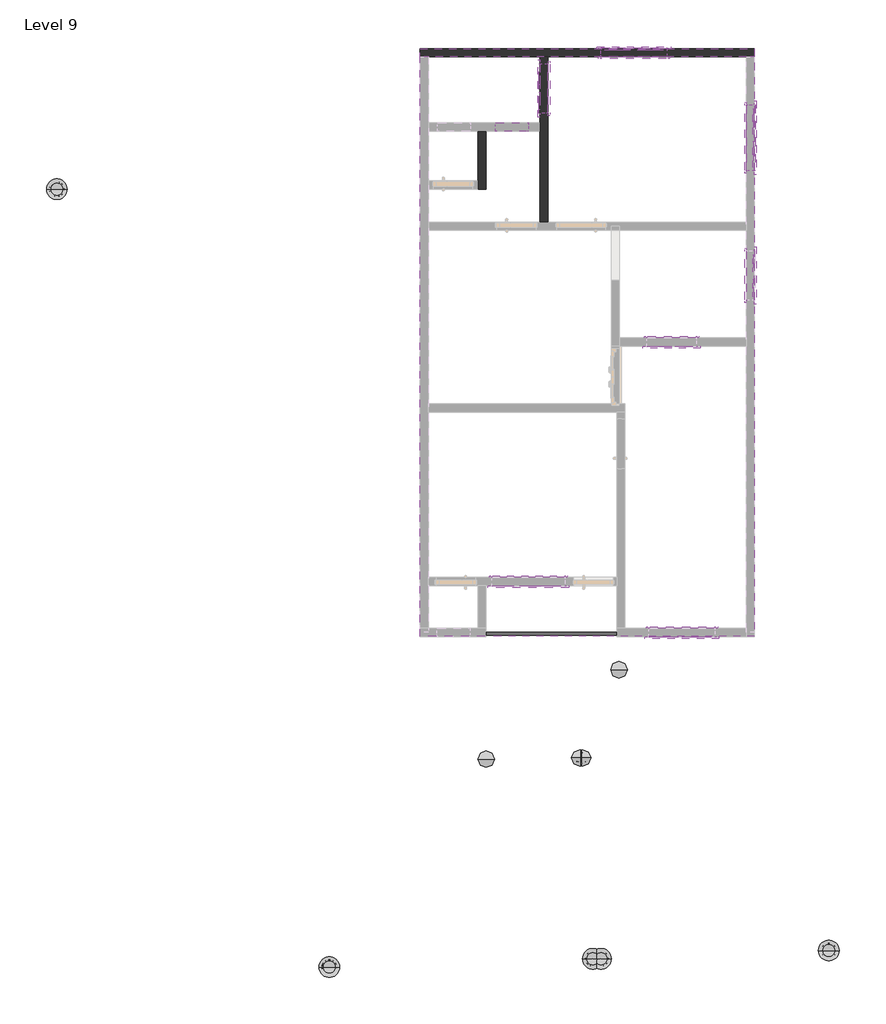
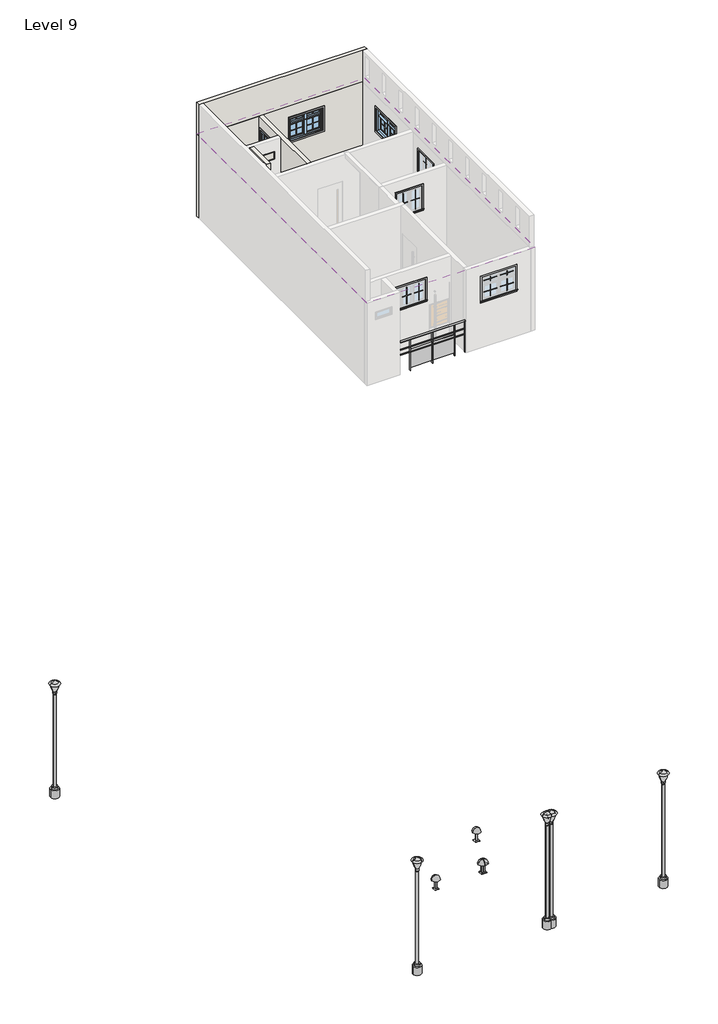
# One storey, part 2 of 2: 48 proxies, 10 light fixtures, 7 walls, 5 windows, 1 covering, 1 railing.
"""IFC4 building model written with IfcOpenShell, lengths in millimetres."""

from ifc_helpers import new_model, si_unit, point, frame, origin, place, context, project, spatial, polyline, ellipse_curve, trimmed, outline, extrude, faceted_brep, transform, mapped, element, save
from ifc_brep_helpers import plane_surface, extruded_surface, advanced_brep
from components import m_muntin_pattern_2x2_m_muntin_pattern_2x2_ec2ff75e, m_muntin_pattern_2x2_m_muntin_pattern_2x2_6a19bea2, m_muntin_pattern_2x2_m_muntin_pattern_2x2_383df7b3, m_muntin_pattern_2x2_m_muntin_pattern_2x2_55460d9e, m_muntin_pattern_2x2_m_muntin_pattern_2x2_a9b7b7a9, m_muntin_pattern_2x2_m_muntin_pattern_2x2_c959817e, m_muntin_pattern_2x2_m_muntin_pattern_2x2_9259c5e2, m_trim_window_exterior_flat_with_sill_b1b88069, m_trim_window_exterior_flat_with_sill_8fa486dc, m_trim_window_exterior_flat_with_sill_2a9c44ae, m_trim_window_interior_flat_picture_frame_7d12f20c, m_trim_window_interior_flat_picture_frame_b6dd03a6, m_trim_window_interior_flat_picture_frame_c139440e, m_street_light_antique_400w_halogen_120v_ac89fb25, m_table_lamp_hemispheric_60w_120v_fef6e77c, fixed_2_65c13adb, m_window_casement_double_3_e0bd8fa3, m_window_casement_double_awning_double_4_7efa9bbd

model = new_model("IFC4")

# Units and contexts
model_context = context("Model", 3, world=origin())
ifc_project = project(units=[si_unit("LENGTHUNIT", "METRE", prefix="MILLI")], contexts=[model_context])

# Site, building, storey
site = spatial("IfcSite", under=ifc_project)
building = spatial("IfcBuilding", under=site)
storey = spatial("IfcBuildingStorey", under=building, Name="Level 9", Elevation=16611.6)

# Proxies
placement = place(None, origin())
m_muntin_pattern_2x2_m_muntin_pattern_2x2_shape = m_muntin_pattern_2x2_m_muntin_pattern_2x2_ec2ff75e(model_context)
element("IfcBuildingElementProxy", 1, Name="M_Muntin Pattern_2x2 : M_Muntin Pattern_2x2", ObjectType="M_Muntin Pattern_2x2 : M_Muntin Pattern_2x2", at=placement, inside=storey, context=model_context, shape_type="MappedRepresentation", body=[
    mapped(m_muntin_pattern_2x2_m_muntin_pattern_2x2_shape, transform((-20164.8088079, 6316.5492053, 18510.25), x_axis=(1.0, 0.0, 0.0), y_axis=(0.0, 1.0, 0.0), z_axis=(0.0, 0.0, 1.0))),
])
element("IfcBuildingElementProxy", 2, Name="M_Muntin Pattern_2x2 : M_Muntin Pattern_2x2", ObjectType="M_Muntin Pattern_2x2 : M_Muntin Pattern_2x2", at=placement, inside=storey, context=model_context, shape_type="MappedRepresentation", body=[
    mapped(m_muntin_pattern_2x2_m_muntin_pattern_2x2_shape, transform((-17648.6213079, 4984.6367053, 18510.25), x_axis=(0.0, -1.0, 0.0), y_axis=(1.0, 0.0, 0.0), z_axis=(0.0, 0.0, 1.0))),
])
element("IfcBuildingElementProxy", 3, Name="M_Muntin Pattern_2x2 : M_Muntin Pattern_2x2", ObjectType="M_Muntin Pattern_2x2 : M_Muntin Pattern_2x2", at=placement, inside=storey, context=model_context, shape_type="MappedRepresentation", body=[
    mapped(m_muntin_pattern_2x2_m_muntin_pattern_2x2_shape, transform((-18672.7572454, -4510.2007947, 18510.25), x_axis=(-1.0, 0.0, 0.0), y_axis=(0.0, -1.0, 0.0), z_axis=(0.0, 0.0, 1.0))),
])
m_muntin_pattern_2x2_m_muntin_pattern_2x2_2_shape = m_muntin_pattern_2x2_m_muntin_pattern_2x2_6a19bea2(model_context)
element("IfcBuildingElementProxy", 4, Name="M_Muntin Pattern_2x2 : M_Muntin Pattern_2x2", ObjectType="M_Muntin Pattern_2x2 : M_Muntin Pattern_2x2", at=placement, inside=storey, context=model_context, shape_type="MappedRepresentation", body=[
    mapped(m_muntin_pattern_2x2_m_muntin_pattern_2x2_2_shape, transform((-19558.3838079, 6316.5492053, 18510.25), x_axis=(-1.0, 0.0, 0.0), y_axis=(0.0, -1.0, 0.0), z_axis=(0.0, 0.0, 1.0))),
])
element("IfcBuildingElementProxy", 5, Name="M_Muntin Pattern_2x2 : M_Muntin Pattern_2x2", ObjectType="M_Muntin Pattern_2x2 : M_Muntin Pattern_2x2", at=placement, inside=storey, context=model_context, shape_type="MappedRepresentation", body=[
    mapped(m_muntin_pattern_2x2_m_muntin_pattern_2x2_2_shape, transform((-17648.6213079, 4378.2117053, 18510.25), x_axis=(0.0, 1.0, 0.0), y_axis=(-1.0, 0.0, 0.0), z_axis=(0.0, 0.0, 1.0))),
])
element("IfcBuildingElementProxy", 6, Name="M_Muntin Pattern_2x2 : M_Muntin Pattern_2x2", ObjectType="M_Muntin Pattern_2x2 : M_Muntin Pattern_2x2", at=placement, inside=storey, context=model_context, shape_type="MappedRepresentation", body=[
    mapped(m_muntin_pattern_2x2_m_muntin_pattern_2x2_2_shape, transform((-19279.1822454, -4510.2007947, 18510.25), x_axis=(1.0, 0.0, 0.0), y_axis=(0.0, 1.0, 0.0), z_axis=(0.0, 0.0, 1.0))),
])
m_muntin_pattern_2x2_m_muntin_pattern_2x2_3_shape = m_muntin_pattern_2x2_m_muntin_pattern_2x2_383df7b3(model_context)
element("IfcBuildingElementProxy", 7, Name="M_Muntin Pattern_2x2 : M_Muntin Pattern_2x2", ObjectType="M_Muntin Pattern_2x2 : M_Muntin Pattern_2x2", at=placement, inside=storey, context=model_context, shape_type="MappedRepresentation", body=[
    mapped(m_muntin_pattern_2x2_m_muntin_pattern_2x2_3_shape, transform((-19558.3838079, 6316.5492053, 19110.25), x_axis=(-1.0, 0.0, 0.0), y_axis=(0.0, -1.0, 0.0), z_axis=(0.0, 0.0, 1.0))),
])
element("IfcBuildingElementProxy", 8, Name="M_Muntin Pattern_2x2 : M_Muntin Pattern_2x2", ObjectType="M_Muntin Pattern_2x2 : M_Muntin Pattern_2x2", at=placement, inside=storey, context=model_context, shape_type="MappedRepresentation", body=[
    mapped(m_muntin_pattern_2x2_m_muntin_pattern_2x2_3_shape, transform((-20164.8088079, 6316.5492053, 19110.25), x_axis=(-1.0, 0.0, 0.0), y_axis=(0.0, -1.0, 0.0), z_axis=(0.0, 0.0, 1.0))),
])
element("IfcBuildingElementProxy", 9, Name="M_Muntin Pattern_2x2 : M_Muntin Pattern_2x2", ObjectType="M_Muntin Pattern_2x2 : M_Muntin Pattern_2x2", at=placement, inside=storey, context=model_context, shape_type="MappedRepresentation", body=[
    mapped(m_muntin_pattern_2x2_m_muntin_pattern_2x2_3_shape, transform((-17648.6213079, 4378.2117053, 19110.25), x_axis=(0.0, 1.0, 0.0), y_axis=(-1.0, 0.0, 0.0), z_axis=(0.0, 0.0, 1.0))),
])
element("IfcBuildingElementProxy", 10, Name="M_Muntin Pattern_2x2 : M_Muntin Pattern_2x2", ObjectType="M_Muntin Pattern_2x2 : M_Muntin Pattern_2x2", at=placement, inside=storey, context=model_context, shape_type="MappedRepresentation", body=[
    mapped(m_muntin_pattern_2x2_m_muntin_pattern_2x2_3_shape, transform((-17648.6213079, 4984.6367053, 19110.25), x_axis=(0.0, 1.0, 0.0), y_axis=(-1.0, 0.0, 0.0), z_axis=(0.0, 0.0, 1.0))),
])
element("IfcBuildingElementProxy", 11, Name="M_Muntin Pattern_2x2 : M_Muntin Pattern_2x2", ObjectType="M_Muntin Pattern_2x2 : M_Muntin Pattern_2x2", at=placement, inside=storey, context=model_context, shape_type="MappedRepresentation", body=[
    mapped(m_muntin_pattern_2x2_m_muntin_pattern_2x2_3_shape, transform((-19279.1822454, -4510.2007947, 19110.25), x_axis=(1.0, 0.0, 0.0), y_axis=(0.0, 1.0, 0.0), z_axis=(0.0, 0.0, 1.0))),
])
element("IfcBuildingElementProxy", 12, Name="M_Muntin Pattern_2x2 : M_Muntin Pattern_2x2", ObjectType="M_Muntin Pattern_2x2 : M_Muntin Pattern_2x2", at=placement, inside=storey, context=model_context, shape_type="MappedRepresentation", body=[
    mapped(m_muntin_pattern_2x2_m_muntin_pattern_2x2_3_shape, transform((-18672.7572454, -4510.2007947, 19110.25), x_axis=(1.0, 0.0, 0.0), y_axis=(0.0, 1.0, 0.0), z_axis=(0.0, 0.0, 1.0))),
])
m_muntin_pattern_2x2_m_muntin_pattern_2x2_4_shape = m_muntin_pattern_2x2_m_muntin_pattern_2x2_55460d9e(model_context)
element("IfcBuildingElementProxy", 13, Name="M_Muntin Pattern_2x2 : M_Muntin Pattern_2x2", ObjectType="M_Muntin Pattern_2x2 : M_Muntin Pattern_2x2", at=placement, inside=storey, context=model_context, shape_type="MappedRepresentation", body=[
    mapped(m_muntin_pattern_2x2_m_muntin_pattern_2x2_4_shape, transform((-18939.9533391, 849.1992053, 18510.25), x_axis=(-1.0, 0.0, 0.0), y_axis=(0.0, -1.0, 0.0), z_axis=(0.0, 0.0, 1.0))),
])
element("IfcBuildingElementProxy", 14, Name="M_Muntin Pattern_2x2 : M_Muntin Pattern_2x2", ObjectType="M_Muntin Pattern_2x2 : M_Muntin Pattern_2x2", at=placement, inside=storey, context=model_context, shape_type="MappedRepresentation", body=[
    mapped(m_muntin_pattern_2x2_m_muntin_pattern_2x2_4_shape, transform((-17648.6213079, 2366.8492053, 18510.25), x_axis=(0.0, -1.0, 0.0), y_axis=(1.0, 0.0, 0.0), z_axis=(0.0, 0.0, 1.0))),
])
element("IfcBuildingElementProxy", 15, Name="M_Muntin Pattern_2x2 : M_Muntin Pattern_2x2", ObjectType="M_Muntin Pattern_2x2 : M_Muntin Pattern_2x2", at=placement, inside=storey, context=model_context, shape_type="MappedRepresentation", body=[
    mapped(m_muntin_pattern_2x2_m_muntin_pattern_2x2_4_shape, transform((-21591.9713079, 5362.4617053, 18510.25), x_axis=(0.0, 1.0, 0.0), y_axis=(-1.0, 0.0, 0.0), z_axis=(0.0, 0.0, 1.0))),
])
element("IfcBuildingElementProxy", 16, Name="M_Muntin Pattern_2x2 : M_Muntin Pattern_2x2", ObjectType="M_Muntin Pattern_2x2 : M_Muntin Pattern_2x2", at=placement, inside=storey, context=model_context, shape_type="MappedRepresentation", body=[
    mapped(m_muntin_pattern_2x2_m_muntin_pattern_2x2_4_shape, transform((-18939.9533391, 849.1992053, 18510.25), x_axis=(-1.0, 0.0, 0.0), y_axis=(0.0, -1.0, 0.0), z_axis=(0.0, 0.0, 1.0))),
])
element("IfcBuildingElementProxy", 17, Name="M_Muntin Pattern_2x2 : M_Muntin Pattern_2x2", ObjectType="M_Muntin Pattern_2x2 : M_Muntin Pattern_2x2", at=placement, inside=storey, context=model_context, shape_type="MappedRepresentation", body=[
    mapped(m_muntin_pattern_2x2_m_muntin_pattern_2x2_4_shape, transform((-21591.9713079, 5362.4617053, 18510.25), x_axis=(0.0, 1.0, 0.0), y_axis=(-1.0, 0.0, 0.0), z_axis=(0.0, 0.0, 1.0))),
])
m_muntin_pattern_2x2_m_muntin_pattern_2x2_5_shape = m_muntin_pattern_2x2_m_muntin_pattern_2x2_a9b7b7a9(model_context)
element("IfcBuildingElementProxy", 18, Name="M_Muntin Pattern_2x2 : M_Muntin Pattern_2x2", ObjectType="M_Muntin Pattern_2x2 : M_Muntin Pattern_2x2", at=placement, inside=storey, context=model_context, shape_type="MappedRepresentation", body=[
    mapped(m_muntin_pattern_2x2_m_muntin_pattern_2x2_5_shape, transform((-19393.9783391, 849.1992053, 18510.25), x_axis=(1.0, 0.0, 0.0), y_axis=(0.0, 1.0, 0.0), z_axis=(0.0, 0.0, 1.0))),
])
element("IfcBuildingElementProxy", 19, Name="M_Muntin Pattern_2x2 : M_Muntin Pattern_2x2", ObjectType="M_Muntin Pattern_2x2 : M_Muntin Pattern_2x2", at=placement, inside=storey, context=model_context, shape_type="MappedRepresentation", body=[
    mapped(m_muntin_pattern_2x2_m_muntin_pattern_2x2_5_shape, transform((-17648.6213079, 1912.8242053, 18510.25), x_axis=(0.0, 1.0, 0.0), y_axis=(-1.0, 0.0, 0.0), z_axis=(0.0, 0.0, 1.0))),
])
element("IfcBuildingElementProxy", 20, Name="M_Muntin Pattern_2x2 : M_Muntin Pattern_2x2", ObjectType="M_Muntin Pattern_2x2 : M_Muntin Pattern_2x2", at=placement, inside=storey, context=model_context, shape_type="MappedRepresentation", body=[
    mapped(m_muntin_pattern_2x2_m_muntin_pattern_2x2_5_shape, transform((-21591.9713079, 5816.4867053, 18510.25), x_axis=(0.0, -1.0, 0.0), y_axis=(1.0, 0.0, 0.0), z_axis=(0.0, 0.0, 1.0))),
])
element("IfcBuildingElementProxy", 21, Name="M_Muntin Pattern_2x2 : M_Muntin Pattern_2x2", ObjectType="M_Muntin Pattern_2x2 : M_Muntin Pattern_2x2", at=placement, inside=storey, context=model_context, shape_type="MappedRepresentation", body=[
    mapped(m_muntin_pattern_2x2_m_muntin_pattern_2x2_5_shape, transform((-19393.9783391, 849.1992053, 18510.25), x_axis=(1.0, 0.0, 0.0), y_axis=(0.0, 1.0, 0.0), z_axis=(0.0, 0.0, 1.0))),
])
element("IfcBuildingElementProxy", 22, Name="M_Muntin Pattern_2x2 : M_Muntin Pattern_2x2", ObjectType="M_Muntin Pattern_2x2 : M_Muntin Pattern_2x2", at=placement, inside=storey, context=model_context, shape_type="MappedRepresentation", body=[
    mapped(m_muntin_pattern_2x2_m_muntin_pattern_2x2_5_shape, transform((-21591.9713079, 5816.4867053, 18510.25), x_axis=(0.0, -1.0, 0.0), y_axis=(1.0, 0.0, 0.0), z_axis=(0.0, 0.0, 1.0))),
])
m_muntin_pattern_2x2_m_muntin_pattern_2x2_6_shape = m_muntin_pattern_2x2_m_muntin_pattern_2x2_c959817e(model_context)
element("IfcBuildingElementProxy", 23, Name="M_Muntin Pattern_2x2 : M_Muntin Pattern_2x2", ObjectType="M_Muntin Pattern_2x2 : M_Muntin Pattern_2x2", at=placement, inside=storey, context=model_context, shape_type="MappedRepresentation", body=[
    mapped(m_muntin_pattern_2x2_m_muntin_pattern_2x2_6_shape, transform((-21364.4296412, -3570.4007947, 18510.25), x_axis=(-1.0, 0.0, 0.0), y_axis=(0.0, -1.0, 0.0), z_axis=(0.0, 0.0, 1.0))),
])
element("IfcBuildingElementProxy", 24, Name="M_Muntin Pattern_2x2 : M_Muntin Pattern_2x2", ObjectType="M_Muntin Pattern_2x2 : M_Muntin Pattern_2x2", at=placement, inside=storey, context=model_context, shape_type="MappedRepresentation", body=[
    mapped(m_muntin_pattern_2x2_m_muntin_pattern_2x2_6_shape, transform((-21364.4296412, -3570.4007947, 18510.25), x_axis=(-1.0, 0.0, 0.0), y_axis=(0.0, -1.0, 0.0), z_axis=(0.0, 0.0, 1.0))),
])
m_muntin_pattern_2x2_m_muntin_pattern_2x2_7_shape = m_muntin_pattern_2x2_m_muntin_pattern_2x2_9259c5e2(model_context)
element("IfcBuildingElementProxy", 25, Name="M_Muntin Pattern_2x2 : M_Muntin Pattern_2x2", ObjectType="M_Muntin Pattern_2x2 : M_Muntin Pattern_2x2", at=placement, inside=storey, context=model_context, shape_type="MappedRepresentation", body=[
    mapped(m_muntin_pattern_2x2_m_muntin_pattern_2x2_7_shape, transform((-22257.6629746, -3570.4007947, 18510.25), x_axis=(1.0, 0.0, 0.0), y_axis=(0.0, 1.0, 0.0), z_axis=(0.0, 0.0, 1.0))),
])
element("IfcBuildingElementProxy", 26, Name="M_Muntin Pattern_2x2 : M_Muntin Pattern_2x2", ObjectType="M_Muntin Pattern_2x2 : M_Muntin Pattern_2x2", at=placement, inside=storey, context=model_context, shape_type="MappedRepresentation", body=[
    mapped(m_muntin_pattern_2x2_m_muntin_pattern_2x2_7_shape, transform((-21811.0463079, -3570.4007947, 18510.25), x_axis=(1.0, 0.0, 0.0), y_axis=(0.0, 1.0, 0.0), z_axis=(0.0, 0.0, 1.0))),
])
element("IfcBuildingElementProxy", 27, Name="M_Muntin Pattern_2x2 : M_Muntin Pattern_2x2", ObjectType="M_Muntin Pattern_2x2 : M_Muntin Pattern_2x2", at=placement, inside=storey, context=model_context, shape_type="MappedRepresentation", body=[
    mapped(m_muntin_pattern_2x2_m_muntin_pattern_2x2_7_shape, transform((-22257.6629746, -3570.4007947, 18510.25), x_axis=(1.0, 0.0, 0.0), y_axis=(0.0, 1.0, 0.0), z_axis=(0.0, 0.0, 1.0))),
])
element("IfcBuildingElementProxy", 28, Name="M_Muntin Pattern_2x2 : M_Muntin Pattern_2x2", ObjectType="M_Muntin Pattern_2x2 : M_Muntin Pattern_2x2", at=placement, inside=storey, context=model_context, shape_type="MappedRepresentation", body=[
    mapped(m_muntin_pattern_2x2_m_muntin_pattern_2x2_7_shape, transform((-21811.0463079, -3570.4007947, 18510.25), x_axis=(1.0, 0.0, 0.0), y_axis=(0.0, 1.0, 0.0), z_axis=(0.0, 0.0, 1.0))),
])
m_trim_window_exterior_flat_with_sill_shape = m_trim_window_exterior_flat_with_sill_b1b88069(model_context)
element("IfcBuildingElementProxy", 29, Name="M_Trim-Window-Exterior-Flat : with Sill", ObjectType="M_Trim-Window-Exterior-Flat : with Sill", at=placement, inside=storey, context=model_context, shape_type="MappedRepresentation", body=[
    mapped(m_trim_window_exterior_flat_with_sill_shape, transform((-19861.5963079, 6326.0742053, 19340.4), x_axis=(-1.0, 0.0, 0.0), y_axis=(0.0, 0.0, 1.0), z_axis=(0.0, 1.0, 0.0))),
])
element("IfcBuildingElementProxy", 30, Name="M_Trim-Window-Exterior-Flat : with Sill", ObjectType="M_Trim-Window-Exterior-Flat : with Sill", at=placement, inside=storey, context=model_context, shape_type="MappedRepresentation", body=[
    mapped(m_trim_window_exterior_flat_with_sill_shape, transform((-17639.0963079, 4681.4242053, 19340.4), x_axis=(0.0, 1.0, 0.0), y_axis=(0.0, 0.0, 1.0), z_axis=(1.0, 0.0, 0.0))),
])
element("IfcBuildingElementProxy", 31, Name="M_Trim-Window-Exterior-Flat : with Sill", ObjectType="M_Trim-Window-Exterior-Flat : with Sill", at=placement, inside=storey, context=model_context, shape_type="MappedRepresentation", body=[
    mapped(m_trim_window_exterior_flat_with_sill_shape, transform((-18975.9697454, -4519.7257947, 19340.4), x_axis=(1.0, 0.0, 0.0), y_axis=(0.0, 0.0, 1.0), z_axis=(0.0, -1.0, 0.0))),
])
m_trim_window_exterior_flat_with_sill_2_shape = m_trim_window_exterior_flat_with_sill_8fa486dc(model_context)
element("IfcBuildingElementProxy", 32, Name="M_Trim-Window-Exterior-Flat : with Sill", ObjectType="M_Trim-Window-Exterior-Flat : with Sill", at=placement, inside=storey, context=model_context, shape_type="MappedRepresentation", body=[
    mapped(m_trim_window_exterior_flat_with_sill_2_shape, transform((-19166.9658391, 839.6742053, 19340.4), x_axis=(1.0, 0.0, 0.0), y_axis=(0.0, 0.0, 1.0), z_axis=(0.0, -1.0, 0.0))),
])
element("IfcBuildingElementProxy", 33, Name="M_Trim-Window-Exterior-Flat : with Sill", ObjectType="M_Trim-Window-Exterior-Flat : with Sill", at=placement, inside=storey, context=model_context, shape_type="MappedRepresentation", body=[
    mapped(m_trim_window_exterior_flat_with_sill_2_shape, transform((-17639.0963079, 2139.8367053, 19340.4), x_axis=(0.0, 1.0, 0.0), y_axis=(0.0, 0.0, 1.0), z_axis=(1.0, 0.0, 0.0))),
])
element("IfcBuildingElementProxy", 34, Name="M_Trim-Window-Exterior-Flat : with Sill", ObjectType="M_Trim-Window-Exterior-Flat : with Sill", at=placement, inside=storey, context=model_context, shape_type="MappedRepresentation", body=[
    mapped(m_trim_window_exterior_flat_with_sill_2_shape, transform((-21601.4963079, 5589.4742053, 19340.4), x_axis=(0.0, -1.0, 0.0), y_axis=(0.0, 0.0, 1.0), z_axis=(-1.0, 0.0, 0.0))),
])
element("IfcBuildingElementProxy", 35, Name="M_Trim-Window-Exterior-Flat : with Sill", ObjectType="M_Trim-Window-Exterior-Flat : with Sill", at=placement, inside=storey, context=model_context, shape_type="MappedRepresentation", body=[
    mapped(m_trim_window_exterior_flat_with_sill_2_shape, transform((-19166.9658391, 839.6742053, 19340.4), x_axis=(1.0, 0.0, 0.0), y_axis=(0.0, 0.0, 1.0), z_axis=(0.0, -1.0, 0.0))),
])
element("IfcBuildingElementProxy", 36, Name="M_Trim-Window-Exterior-Flat : with Sill", ObjectType="M_Trim-Window-Exterior-Flat : with Sill", at=placement, inside=storey, context=model_context, shape_type="MappedRepresentation", body=[
    mapped(m_trim_window_exterior_flat_with_sill_2_shape, transform((-21601.4963079, 5589.4742053, 19340.4), x_axis=(0.0, -1.0, 0.0), y_axis=(0.0, 0.0, 1.0), z_axis=(-1.0, 0.0, 0.0))),
])
m_trim_window_exterior_flat_with_sill_3_shape = m_trim_window_exterior_flat_with_sill_2a9c44ae(model_context)
element("IfcBuildingElementProxy", 37, Name="M_Trim-Window-Exterior-Flat : with Sill", ObjectType="M_Trim-Window-Exterior-Flat : with Sill", at=placement, inside=storey, context=model_context, shape_type="MappedRepresentation", body=[
    mapped(m_trim_window_exterior_flat_with_sill_3_shape, transform((-21811.0463079, -3579.9257947, 19240.4), x_axis=(1.0, 0.0, 0.0), y_axis=(0.0, 0.0, 1.0), z_axis=(0.0, -1.0, 0.0))),
])
element("IfcBuildingElementProxy", 38, Name="M_Trim-Window-Exterior-Flat : with Sill", ObjectType="M_Trim-Window-Exterior-Flat : with Sill", at=placement, inside=storey, context=model_context, shape_type="MappedRepresentation", body=[
    mapped(m_trim_window_exterior_flat_with_sill_3_shape, transform((-21811.0463079, -3579.9257947, 19240.4), x_axis=(1.0, 0.0, 0.0), y_axis=(0.0, 0.0, 1.0), z_axis=(0.0, -1.0, 0.0))),
])
m_trim_window_interior_flat_picture_frame_shape = m_trim_window_interior_flat_picture_frame_7d12f20c(model_context)
element("IfcBuildingElementProxy", 39, Name="M_Trim-Window-Interior-Flat : Picture Frame", ObjectType="M_Trim-Window-Interior-Flat : Picture Frame", at=placement, inside=storey, context=model_context, shape_type="MappedRepresentation", body=[
    mapped(m_trim_window_interior_flat_picture_frame_shape, transform((-19861.5963079, 6173.6742053, 19340.4), x_axis=(1.0, 0.0, 0.0), y_axis=(0.0, 0.0, 1.0), z_axis=(0.0, -1.0, 0.0))),
])
element("IfcBuildingElementProxy", 40, Name="M_Trim-Window-Interior-Flat : Picture Frame", ObjectType="M_Trim-Window-Interior-Flat : Picture Frame", at=placement, inside=storey, context=model_context, shape_type="MappedRepresentation", body=[
    mapped(m_trim_window_interior_flat_picture_frame_shape, transform((-17791.4963079, 4681.4242053, 19340.4), x_axis=(0.0, -1.0, 0.0), y_axis=(0.0, 0.0, 1.0), z_axis=(-1.0, 0.0, 0.0))),
])
element("IfcBuildingElementProxy", 41, Name="M_Trim-Window-Interior-Flat : Picture Frame", ObjectType="M_Trim-Window-Interior-Flat : Picture Frame", at=placement, inside=storey, context=model_context, shape_type="MappedRepresentation", body=[
    mapped(m_trim_window_interior_flat_picture_frame_shape, transform((-18975.9697454, -4367.3257947, 19340.4), x_axis=(-1.0, 0.0, 0.0), y_axis=(0.0, 0.0, 1.0), z_axis=(0.0, 1.0, 0.0))),
])
m_trim_window_interior_flat_picture_frame_2_shape = m_trim_window_interior_flat_picture_frame_b6dd03a6(model_context)
element("IfcBuildingElementProxy", 42, Name="M_Trim-Window-Interior-Flat : Picture Frame", ObjectType="M_Trim-Window-Interior-Flat : Picture Frame", at=placement, inside=storey, context=model_context, shape_type="MappedRepresentation", body=[
    mapped(m_trim_window_interior_flat_picture_frame_2_shape, transform((-19166.9658391, 992.0742053, 19340.4), x_axis=(-1.0, 0.0, 0.0), y_axis=(0.0, 0.0, 1.0), z_axis=(0.0, 1.0, 0.0))),
])
element("IfcBuildingElementProxy", 43, Name="M_Trim-Window-Interior-Flat : Picture Frame", ObjectType="M_Trim-Window-Interior-Flat : Picture Frame", at=placement, inside=storey, context=model_context, shape_type="MappedRepresentation", body=[
    mapped(m_trim_window_interior_flat_picture_frame_2_shape, transform((-17791.4963079, 2139.8367053, 19340.4), x_axis=(0.0, -1.0, 0.0), y_axis=(0.0, 0.0, 1.0), z_axis=(-1.0, 0.0, 0.0))),
])
element("IfcBuildingElementProxy", 44, Name="M_Trim-Window-Interior-Flat : Picture Frame", ObjectType="M_Trim-Window-Interior-Flat : Picture Frame", at=placement, inside=storey, context=model_context, shape_type="MappedRepresentation", body=[
    mapped(m_trim_window_interior_flat_picture_frame_2_shape, transform((-21449.0963079, 5589.4742053, 19340.4), x_axis=(0.0, 1.0, 0.0), y_axis=(0.0, 0.0, 1.0), z_axis=(1.0, 0.0, 0.0))),
])
element("IfcBuildingElementProxy", 45, Name="M_Trim-Window-Interior-Flat : Picture Frame", ObjectType="M_Trim-Window-Interior-Flat : Picture Frame", at=placement, inside=storey, context=model_context, shape_type="MappedRepresentation", body=[
    mapped(m_trim_window_interior_flat_picture_frame_2_shape, transform((-19166.9658391, 992.0742053, 19340.4), x_axis=(-1.0, 0.0, 0.0), y_axis=(0.0, 0.0, 1.0), z_axis=(0.0, 1.0, 0.0))),
])
element("IfcBuildingElementProxy", 46, Name="M_Trim-Window-Interior-Flat : Picture Frame", ObjectType="M_Trim-Window-Interior-Flat : Picture Frame", at=placement, inside=storey, context=model_context, shape_type="MappedRepresentation", body=[
    mapped(m_trim_window_interior_flat_picture_frame_2_shape, transform((-21449.0963079, 5589.4742053, 19340.4), x_axis=(0.0, 1.0, 0.0), y_axis=(0.0, 0.0, 1.0), z_axis=(1.0, 0.0, 0.0))),
])
m_trim_window_interior_flat_picture_frame_3_shape = m_trim_window_interior_flat_picture_frame_c139440e(model_context)
element("IfcBuildingElementProxy", 47, Name="M_Trim-Window-Interior-Flat : Picture Frame", ObjectType="M_Trim-Window-Interior-Flat : Picture Frame", at=placement, inside=storey, context=model_context, shape_type="MappedRepresentation", body=[
    mapped(m_trim_window_interior_flat_picture_frame_3_shape, transform((-21811.0463079, -3427.5257947, 19240.4), x_axis=(-1.0, 0.0, 0.0), y_axis=(0.0, 0.0, 1.0), z_axis=(0.0, 1.0, 0.0))),
])
element("IfcBuildingElementProxy", 48, Name="M_Trim-Window-Interior-Flat : Picture Frame", ObjectType="M_Trim-Window-Interior-Flat : Picture Frame", at=placement, inside=storey, context=model_context, shape_type="MappedRepresentation", body=[
    mapped(m_trim_window_interior_flat_picture_frame_3_shape, transform((-21811.0463079, -3427.5257947, 19240.4), x_axis=(-1.0, 0.0, 0.0), y_axis=(0.0, 0.0, 1.0), z_axis=(0.0, 1.0, 0.0))),
])

# Covering
element("IfcCovering", 49, ObjectType="2' x 4' ACT System", at=placement, inside=storey, context=model_context, shape_type="SweptSolid", body=[
    extrude(outline(polyline([(-23811.2963079, -4519.7257947), (-23811.2963079, 6326.0742053), (-17639.0963079, 6326.0742053), (-17639.0963079, -4519.7257947), (-22309.2664727, -4519.7257947), (-23811.2963079, -4519.7257947)])), frame((0.0, 0.0, 19812.0), z_axis=(0.0, 0.0, 1.0), x_axis=(1.0, 0.0, 0.0)), (0.0, 0.0, 1.0), 57.15),
])

# Light fixtures
m_street_light_antique_400w_halogen_120v_shape = m_street_light_antique_400w_halogen_120v_ac89fb25(model_context)
element("IfcLightFixture", 50, ObjectType="M_Street Light - Antique : 400W Halogen - 120V", at=placement, inside=storey, context=model_context, shape_type="MappedRepresentation", body=[
    mapped(m_street_light_antique_400w_halogen_120v_shape, transform((-16267.4963079, -10310.2685721, -1936.0232956), x_axis=(1.0, 0.0, 0.0), y_axis=(0.0, 1.0, 0.0), z_axis=(0.0, 0.0, 1.0))),
])
element("IfcLightFixture", 51, ObjectType="M_Street Light - Antique : 400W Halogen - 120V", at=placement, inside=storey, context=model_context, shape_type="MappedRepresentation", body=[
    mapped(m_street_light_antique_400w_halogen_120v_shape, transform((-20471.1963079, -10462.8323892, -1917.9019302), x_axis=(1.0, 0.0, 0.0), y_axis=(0.0, 1.0, 0.0), z_axis=(0.0, 0.0, 1.0))),
])
element("IfcLightFixture", 52, ObjectType="M_Street Light - Antique : 400W Halogen - 120V", at=placement, inside=storey, context=model_context, shape_type="MappedRepresentation", body=[
    mapped(m_street_light_antique_400w_halogen_120v_shape, transform((-20623.5963079, -10462.8323892, -1917.9019302), x_axis=(1.0, 0.0, 0.0), y_axis=(0.0, 1.0, 0.0), z_axis=(0.0, 0.0, 1.0))),
])
element("IfcLightFixture", 53, ObjectType="M_Street Light - Antique : 400W Halogen - 120V", at=placement, inside=storey, context=model_context, shape_type="MappedRepresentation", body=[
    mapped(m_street_light_antique_400w_halogen_120v_shape, transform((-25487.6963079, -10615.7175512, -1899.7423958), x_axis=(1.0, 0.0, 0.0), y_axis=(0.0, 1.0, 0.0), z_axis=(0.0, 0.0, 1.0))),
])
element("IfcLightFixture", 54, ObjectType="M_Street Light - Antique : 400W Halogen - 120V", at=placement, inside=storey, context=model_context, shape_type="MappedRepresentation", body=[
    mapped(m_street_light_antique_400w_halogen_120v_shape, transform((-30516.8963079, 3735.2742053, -1981.2), x_axis=(1.0, 0.0, 0.0), y_axis=(0.0, 1.0, 0.0), z_axis=(0.0, 0.0, 1.0))),
])
m_table_lamp_hemispheric_60w_120v_shape = m_table_lamp_hemispheric_60w_120v_fef6e77c(model_context)
element("IfcLightFixture", 55, ObjectType="M_Table Lamp - Hemispheric : 60W - 120V", at=placement, inside=storey, context=model_context, shape_type="MappedRepresentation", body=[
    mapped(m_table_lamp_hemispheric_60w_120v_shape, transform((-22592.0963079, -6780.3257947, -1981.2), x_axis=(1.0, 0.0, 0.0), y_axis=(0.0, 1.0, 0.0), z_axis=(0.0, 0.0, 1.0))),
])
element("IfcLightFixture", 56, ObjectType="M_Table Lamp - Hemispheric : 60W - 120V", at=placement, inside=storey, context=model_context, shape_type="MappedRepresentation", body=[
    mapped(m_table_lamp_hemispheric_60w_120v_shape, transform((-20864.8963079, -6754.9257947, -1981.2), x_axis=(1.0, 0.0, 0.0), y_axis=(0.0, 1.0, 0.0), z_axis=(0.0, 0.0, 1.0))),
])
element("IfcLightFixture", 57, ObjectType="M_Table Lamp - Hemispheric : 60W - 120V", at=placement, inside=storey, context=model_context, shape_type="MappedRepresentation", body=[
    mapped(m_table_lamp_hemispheric_60w_120v_shape, transform((-20814.0963079, -6754.9257947, -1981.2), x_axis=(1.0, 0.0, 0.0), y_axis=(0.0, 1.0, 0.0), z_axis=(0.0, 0.0, 1.0))),
])
element("IfcLightFixture", 58, ObjectType="M_Table Lamp - Hemispheric : 60W - 120V", at=placement, inside=storey, context=model_context, shape_type="MappedRepresentation", body=[
    mapped(m_table_lamp_hemispheric_60w_120v_shape, transform((-20839.4963079, -6754.9257947, -1981.2), x_axis=(1.0, 0.0, 0.0), y_axis=(0.0, 1.0, 0.0), z_axis=(0.0, 0.0, 1.0))),
])
element("IfcLightFixture", 59, ObjectType="M_Table Lamp - Hemispheric : 60W - 120V", at=placement, inside=storey, context=model_context, shape_type="MappedRepresentation", body=[
    mapped(m_table_lamp_hemispheric_60w_120v_shape, transform((-20140.9963079, -5129.3257947, -1981.2), x_axis=(1.0, 0.0, 0.0), y_axis=(0.0, 1.0, 0.0), z_axis=(0.0, 0.0, 1.0))),
])

# Railing
element("IfcRailing", 60, ObjectType="Glass Panel - Bottom Fill", at=placement, inside=storey, context=model_context, shape_type="SolidModel", body=[
    advanced_brep(
    [(-22592.0963079, -4430.8257947, 17830.8), (-22592.0963079, -4507.0257947, 17830.8), (-20179.0963079, -4430.8257947, 17830.8), (-20179.0963079, -4507.0257947, 17830.8)],
    [
        (0, 1, ellipse_curve(frame((-22592.0963079, -4468.9257947, 17830.8), z_axis=(-1.0, 0.0, 0.0), x_axis=(0.0, -1.0, 0.0)), 38.1, 28.575)),
        (1, 0, ellipse_curve(frame((-22592.0963079, -4468.9257947, 17830.8), z_axis=(-1.0, 0.0, 0.0), x_axis=(0.0, -1.0, 0.0)), 38.1, 28.575)),
        (2, 3, ellipse_curve(frame((-20179.0963079, -4468.9257947, 17830.8), z_axis=(1.0, 0.0, 0.0), x_axis=(0.0, -1.0, 0.0)), 38.1, 28.575)),
        (3, 2, ellipse_curve(frame((-20179.0963079, -4468.9257947, 17830.8), z_axis=(1.0, 0.0, 0.0), x_axis=(0.0, -1.0, 0.0)), 38.1, 28.575)),
        (0, 2),
        (3, 1),
    ],
    [
        plane_surface(frame((-22592.0963079, -4468.9257947, 17830.8), z_axis=(-1.0, 0.0, 0.0), x_axis=(0.0, 1.0, 0.0))),
        plane_surface(frame((-20179.0963079, -4468.9257947, 17830.8), z_axis=(1.0, 0.0, 0.0), x_axis=(0.0, 1.0, 0.0))),
        extruded_surface(trimmed(ellipse_curve(frame((-20179.0963079, -4468.9257947, 17830.8), z_axis=(-1.0, 0.0, 0.0), x_axis=(0.0, -1.0, 0.0)), 38.1, 28.575), [point((-20179.0963079, -4430.8257947, 17830.8))], [point((-20179.0963079, -4507.0257947, 17830.8))], True, "CARTESIAN"), (-2413.0, 0.0, 0.0), 2413.0),
        extruded_surface(trimmed(ellipse_curve(frame((-20179.0963079, -4468.9257947, 17830.8), z_axis=(-1.0, 0.0, 0.0), x_axis=(0.0, -1.0, 0.0)), 38.1, 28.575), [point((-20179.0963079, -4507.0257947, 17830.8))], [point((-20179.0963079, -4430.8257947, 17830.8))], True, "CARTESIAN"), (-2413.0, 0.0, 0.0), 2413.0),
    ],
    [
        (0, [[1, 2]]),
        (1, [[3, 4]]),
        (2, [[-1, 5, -4, 6]]),
        (3, [[-2, -6, -3, -5]]),
    ],
),
    extrude(outline(polyline([(-22592.0963079, -4481.6257947), (-22592.0963079, -4456.2257947), (-20179.0963079, -4456.2257947), (-20179.0963079, -4481.6257947), (-22592.0963079, -4481.6257947)])), frame((0.0, 0.0, 17513.3), z_axis=(0.0, 0.0, 1.0), x_axis=(1.0, 0.0, 0.0)), (0.0, 0.0, 1.0), 25.4),
    extrude(outline(polyline([(-22592.0963079, -4481.6257947), (-22592.0963079, -4456.2257947), (-20179.0963079, -4456.2257947), (-20179.0963079, -4481.6257947), (-22592.0963079, -4481.6257947)])), frame((0.0, 0.0, 17310.1), z_axis=(0.0, 0.0, 1.0), x_axis=(1.0, 0.0, 0.0)), (0.0, 0.0, 1.0), 25.4),
    extrude(outline(polyline([(-20579.1463079, -4494.3257947), (-20579.1463079, -4443.5257947), (-20566.4463079, -4443.5257947), (-20566.4463079, -4494.3257947), (-20579.1463079, -4494.3257947)])), frame((0.0, 0.0, 16611.6), z_axis=(0.0, 0.0, 1.0), x_axis=(1.0, 0.0, 0.0)), (0.0, 0.0, 1.0), 1190.625),
    extrude(outline(polyline([(-21385.5963079, -4462.3906377), (-20572.7963079, -4462.3906377), (-20572.7963079, -4468.7406377), (-21385.5963079, -4468.7406377), (-21385.5963079, -4462.3906377)])), frame((0.0, 0.0, 16713.2), z_axis=(0.0, 0.0, 1.0), x_axis=(1.0, 0.0, 0.0)), (0.0, 0.0, 1.0), 711.2),
    extrude(outline(polyline([(-21391.9463079, -4494.3257947), (-21391.9463079, -4443.5257947), (-21379.2463079, -4443.5257947), (-21379.2463079, -4494.3257947), (-21391.9463079, -4494.3257947)])), frame((0.0, 0.0, 16611.6), z_axis=(0.0, 0.0, 1.0), x_axis=(1.0, 0.0, 0.0)), (0.0, 0.0, 1.0), 1190.625),
    extrude(outline(polyline([(-22198.3963079, -4462.3906377), (-21385.5963079, -4462.3906377), (-21385.5963079, -4468.7406377), (-22198.3963079, -4468.7406377), (-22198.3963079, -4462.3906377)])), frame((0.0, 0.0, 16713.2), z_axis=(0.0, 0.0, 1.0), x_axis=(1.0, 0.0, 0.0)), (0.0, 0.0, 1.0), 711.2),
    extrude(outline(polyline([(-22204.7463079, -4494.3257947), (-22204.7463079, -4443.5257947), (-22192.0463079, -4443.5257947), (-22192.0463079, -4494.3257947), (-22204.7463079, -4494.3257947)])), frame((0.0, 0.0, 16611.6), z_axis=(0.0, 0.0, 1.0), x_axis=(1.0, 0.0, 0.0)), (0.0, 0.0, 1.0), 1190.625),
    extrude(outline(polyline([(-20191.7963079, -4478.4507947), (-20191.7963079, -4459.4007947), (-20172.7463079, -4459.4007947), (-20172.7463079, -4478.4507947), (-20191.7963079, -4478.4507947)])), frame((0.0, 0.0, 16611.6), z_axis=(0.0, 0.0, 1.0), x_axis=(1.0, 0.0, 0.0)), (0.0, 0.0, 1.0), 1190.625),
    extrude(outline(polyline([(-22598.4463079, -4478.4507947), (-22598.4463079, -4459.4007947), (-22579.3963079, -4459.4007947), (-22579.3963079, -4478.4507947), (-22598.4463079, -4478.4507947)])), frame((0.0, 0.0, 16611.6), z_axis=(0.0, 0.0, 1.0), x_axis=(1.0, 0.0, 0.0)), (0.0, 0.0, 1.0), 1190.625),
])

# Walls
element("IfcWall", 61, ObjectType="Generic - 6\"", at=placement, inside=storey, context=model_context, shape_type="Brep", body=[
    faceted_brep([(-23811.2963079, 6173.6742053, 16611.6), (-23658.8963079, 6173.6742053, 16611.6), (-21601.4963079, 6173.6742053, 16611.6), (-21449.0963079, 6173.6742053, 16611.6), (-17791.4963079, 6173.6742053, 16611.6), (-17639.0963079, 6173.6742053, 16611.6), (-17639.0963079, 6173.6742053, 19812.0), (-17791.4963079, 6173.6742053, 19812.0), (-21449.0963079, 6173.6742053, 19812.0), (-21601.4963079, 6173.6742053, 19812.0), (-23658.8963079, 6173.6742053, 19812.0), (-23811.2963079, 6173.6742053, 19812.0), (-19251.9963079, 6173.6742053, 19340.4), (-19251.9963079, 6173.6742053, 18440.4), (-20471.1963079, 6173.6742053, 18440.4), (-20471.1963079, 6173.6742053, 19340.4), (-23811.2963079, 6326.0742053, 16611.6), (-23811.2963079, 6326.0742053, 19812.0), (-17639.0963079, 6326.0742053, 19812.0), (-17639.0963079, 6326.0742053, 16611.6), (-19251.9963079, 6326.0742053, 19340.4), (-20471.1963079, 6326.0742053, 19340.4), (-20471.1963079, 6326.0742053, 18440.4), (-19251.9963079, 6326.0742053, 18440.4)], [[[0, 1, 2, 3, 4, 5, 6, 7, 8, 9, 10, 11], [12, 13, 14, 15]], [[16, 17, 18, 19], [20, 21, 22, 23]], [[5, 4, 3, 2, 1, 0, 16, 19]], [[11, 10, 9, 8, 7, 6, 18, 17]], [[6, 5, 19, 18]], [[0, 11, 17, 16]], [[13, 12, 20, 23]], [[14, 13, 23, 22]], [[15, 14, 22, 21]], [[12, 15, 21, 20]]]),
])
element("IfcWall", 62, ObjectType="Generic - 6\"", at=placement, inside=storey, context=model_context, shape_type="Brep", body=[
    faceted_brep([(-21601.4963079, 6173.6742053, 16611.6), (-21601.4963079, 4954.4742053, 16611.6), (-21601.4963079, 4802.0742053, 16611.6), (-21601.4963079, 3125.6742053, 16611.6), (-21601.4963079, 3125.6742053, 19812.0), (-21601.4963079, 4802.0742053, 19812.0), (-21601.4963079, 4954.4742053, 19812.0), (-21601.4963079, 6173.6742053, 19812.0), (-21601.4963079, 6046.6742053, 19340.4), (-21601.4963079, 5132.2742053, 19340.4), (-21601.4963079, 5132.2742053, 18440.4), (-21601.4963079, 6046.6742053, 18440.4), (-21449.0963079, 6173.6742053, 16611.6), (-21449.0963079, 6173.6742053, 19812.0), (-21449.0963079, 3125.6742053, 19812.0), (-21449.0963079, 3125.6742053, 16611.6), (-21449.0963079, 6046.6742053, 19340.4), (-21449.0963079, 6046.6742053, 18440.4), (-21449.0963079, 5132.2742053, 18440.4), (-21449.0963079, 5132.2742053, 19340.4)], [[[0, 1, 2, 3, 4, 5, 6, 7], [8, 9, 10, 11]], [[12, 13, 14, 15], [16, 17, 18, 19]], [[3, 2, 1, 0, 12, 15]], [[7, 6, 5, 4, 14, 13]], [[0, 7, 13, 12]], [[4, 3, 15, 14]], [[17, 16, 8, 11]], [[18, 17, 11, 10]], [[19, 18, 10, 9]], [[16, 19, 9, 8]]]),
])
element("IfcWall", 63, ObjectType="Generic - 6\"", at=placement, inside=storey, context=model_context, shape_type="Brep", body=[
    faceted_brep([(-22744.4963079, 4802.0742053, 16611.6), (-22744.4963079, 3887.6742053, 16611.6), (-22744.4963079, 3735.2742053, 16611.6), (-22744.4963079, 3735.2742053, 19812.0), (-22744.4963079, 3887.6742053, 19812.0), (-22744.4963079, 4802.0742053, 19812.0), (-22592.0963079, 4802.0742053, 16611.6), (-22592.0963079, 4802.0742053, 19812.0), (-22592.0963079, 3735.2742053, 19812.0), (-22592.0963079, 3735.2742053, 16611.6)], [[[0, 1, 2, 3, 4, 5]], [[6, 7, 8, 9]], [[2, 1, 0, 6, 9]], [[5, 4, 3, 8, 7]], [[0, 5, 7, 6]], [[3, 2, 9, 8]]]),
])
element("IfcWall", 64, ObjectType="Generic - 6\"", at=placement, inside=storey, context=model_context, shape_type="Brep", body=[
    faceted_brep([(-21601.4963079, 6173.6742053, 16611.6), (-21601.4963079, 4954.4742053, 16611.6), (-21601.4963079, 4802.0742053, 16611.6), (-21601.4963079, 3125.6742053, 16611.6), (-21601.4963079, 3125.6742053, 19812.0), (-21601.4963079, 4802.0742053, 19812.0), (-21601.4963079, 4954.4742053, 19812.0), (-21601.4963079, 6173.6742053, 19812.0), (-21601.4963079, 6046.6742053, 19340.4), (-21601.4963079, 5132.2742053, 19340.4), (-21601.4963079, 5132.2742053, 18440.4), (-21601.4963079, 6046.6742053, 18440.4), (-21449.0963079, 6173.6742053, 16611.6), (-21449.0963079, 6173.6742053, 19812.0), (-21449.0963079, 3125.6742053, 19812.0), (-21449.0963079, 3125.6742053, 16611.6), (-21449.0963079, 6046.6742053, 19340.4), (-21449.0963079, 6046.6742053, 18440.4), (-21449.0963079, 5132.2742053, 18440.4), (-21449.0963079, 5132.2742053, 19340.4)], [[[0, 1, 2, 3, 4, 5, 6, 7], [8, 9, 10, 11]], [[12, 13, 14, 15], [16, 17, 18, 19]], [[3, 2, 1, 0, 12, 15]], [[7, 6, 5, 4, 14, 13]], [[4, 3, 15, 14]], [[17, 16, 8, 11]], [[18, 17, 11, 10]], [[19, 18, 10, 9]], [[16, 19, 9, 8]], [[0, 7, 13, 12]]]),
])
element("IfcWall", 65, ObjectType="Generic - 6\"", at=placement, inside=storey, context=model_context, shape_type="Brep", body=[
    faceted_brep([(-23658.8963079, 4802.0742053, 16611.6), (-22744.4963079, 4802.0742053, 16611.6), (-22592.0963079, 4802.0742053, 16611.6), (-21601.4963079, 4802.0742053, 16611.6), (-21601.4963079, 4802.0742053, 19812.0), (-22592.0963079, 4802.0742053, 19812.0), (-22744.4963079, 4802.0742053, 19812.0), (-23658.8963079, 4802.0742053, 19812.0), (-23658.8963079, 4954.4742053, 16611.6), (-23658.8963079, 4954.4742053, 19812.0), (-21601.4963079, 4954.4742053, 19812.0), (-21601.4963079, 4954.4742053, 16611.6)], [[[0, 1, 2, 3, 4, 5, 6, 7]], [[8, 9, 10, 11]], [[3, 2, 1, 0, 8, 11]], [[7, 6, 5, 4, 10, 9]], [[4, 3, 11, 10]], [[0, 7, 9, 8]]]),
])
element("IfcWall", 66, ObjectType="Generic - 6\"", at=placement, inside=storey, context=model_context, shape_type="SweptSolid", body=[
    extrude(outline(polyline([(-22744.4963079, 3887.6742053), (-22744.4963079, 4802.0742053), (-22592.0963079, 4802.0742053), (-22592.0963079, 3887.6742053), (-22744.4963079, 3887.6742053)])), frame((0.0, 0.0, 16611.6), z_axis=(0.0, 0.0, 1.0), x_axis=(1.0, 0.0, 0.0)), (0.0, 0.0, 1.0), 3200.4),
])
element("IfcWall", 67, ObjectType="Generic - 6\"", at=placement, inside=storey, context=model_context, shape_type="Brep", body=[
    faceted_brep([(-23811.2963079, 6173.6742053, 19812.0), (-23658.8963079, 6173.6742053, 19812.0), (-17791.4963079, 6173.6742053, 19812.0), (-17639.0963079, 6173.6742053, 19812.0), (-17639.0963079, 6173.6742053, 21031.2), (-17791.4963079, 6173.6742053, 21031.2), (-23658.8963079, 6173.6742053, 21031.2), (-23811.2963079, 6173.6742053, 21031.2), (-23811.2963079, 6326.0742053, 19812.0), (-23811.2963079, 6326.0742053, 21031.2), (-17639.0963079, 6326.0742053, 21031.2), (-17639.0963079, 6326.0742053, 19812.0)], [[[0, 1, 2, 3, 4, 5, 6, 7]], [[8, 9, 10, 11]], [[3, 2, 1, 0, 8, 11]], [[7, 6, 5, 4, 10, 9]], [[0, 7, 9, 8]], [[4, 3, 11, 10]]]),
])

# Windows
fixed_2_shape = fixed_2_65c13adb(model_context)
element("IfcWindow", 68, ObjectType="Fixed : 2'", at=placement, inside=storey, context=model_context, shape_type="MappedRepresentation", body=[
    mapped(fixed_2_shape, transform((-22079.3338079, 4878.2742053, 18135.6), x_axis=(1.0, 0.0, 0.0), y_axis=(0.0, 1.0, 0.0), z_axis=(0.0, 0.0, 1.0))),
])
m_window_casement_double_3_shape = m_window_casement_double_3_e0bd8fa3(model_context)
element("IfcWindow", 69, ObjectType="M_Window-Casement-Double : 3'", at=placement, inside=storey, context=model_context, shape_type="MappedRepresentation", body=[
    mapped(m_window_casement_double_3_shape, transform((-21525.2963079, 5589.4742053, 17540.4), x_axis=(0.0, 1.0, 0.0), y_axis=(-1.0, 0.0, 0.0), z_axis=(0.0, 0.0, 1.0))),
])
element("IfcWindow", 70, ObjectType="M_Window-Casement-Double : 3'", at=placement, inside=storey, context=model_context, shape_type="MappedRepresentation", body=[
    mapped(m_window_casement_double_3_shape, transform((-21525.2963079, 5589.4742053, 17540.4), x_axis=(0.0, 1.0, 0.0), y_axis=(-1.0, 0.0, 0.0), z_axis=(0.0, 0.0, 1.0))),
])
m_window_casement_double_awning_double_4_shape = m_window_casement_double_awning_double_4_7efa9bbd(model_context)
element("IfcWindow", 71, ObjectType="M_Window-Casement-Double-Awning-Double : 4'", at=placement, inside=storey, context=model_context, shape_type="MappedRepresentation", body=[
    mapped(m_window_casement_double_awning_double_4_shape, transform((-19861.5963079, 6249.8742053, 17540.4), x_axis=(1.0, 0.0, 0.0), y_axis=(0.0, 1.0, 0.0), z_axis=(0.0, 0.0, 1.0))),
])
element("IfcWindow", 72, ObjectType="M_Window-Casement-Double-Awning-Double : 4'", at=placement, inside=storey, context=model_context, shape_type="MappedRepresentation", body=[
    mapped(m_window_casement_double_awning_double_4_shape, transform((-17715.2963079, 4681.4242053, 17540.4), x_axis=(0.0, -1.0, 0.0), y_axis=(1.0, 0.0, 0.0), z_axis=(0.0, 0.0, 1.0))),
])

save(model, "model.ifc")

# Revit data of these elements
# Type "M_Muntin Pattern_2x2 : M_Muntin Pattern_2x2"
#   Width [instance default] = 3' - 11.24409"
#   Thickness = 0' - 0 1/2"
#   Height [instance default] = 3' - 11.24409"
#   Distance = 0' - 0 3/4"
#   Interior Material [instance default] = none
#   Exterior Material [instance default] = none
#   Default Elevation = 0
# Type "M_Trim-Window-Exterior-Flat : with Sill"
#   Trim Width = 0' - 2.3622"
#   Trim Thickness_Picture Frame = 0' - 1.1811"
#   Trim Thickness_with Sill = 0' - 0 3/4"
#   Sill Thickness = 0' - 1.1811"
#   Opening Width [instance default] = 1' - 11.62205"
#   Opening Height [instance default] = 2' - 11.43307"
#   Default Elevation = 3' - 11.24409"
#   Sill = yes
#   Picture Frame = no
#   Trim Material [instance default] = none
# Type "M_Trim-Window-Interior-Flat : Picture Frame"
#   Trim Thickness_Picture Frame = 0' - 1.1811"
#   Trim Width = 0' - 2.3622"
#   Trim Thickness_with Sill = 0' - 0.7874"
#   Sill Thickness = 0' - 1.1811"
#   Opening Width [instance default] = 1' - 11.62205"
#   Opening Height [instance default] = 2' - 11.43307"
#   Default Elevation = 3' - 11.24409"
#   Sill = no
#   Picture Frame = yes
#   Trim Material [instance default] = none
# Type "2' x 4' ACT System"
#   Assembly Code = "C3030210"
#   built-in parameter 1002203 = 1 (stored number, unit not read)
#   built-in parameter 1002202 = 1 (stored number, unit not read)
#   Layers, outside or top first: 0' - 1 5/8" "Default" (function 1); 0' - 0 5/8" "Acoustic Ceiling Tile 24 x 48" (function 5)
# Type "M_Street Light - Antique : 400W Halogen - 120V"
#   Photometric Web File = "SLS1T3.ies"
#   Assembly Code = "D5020280"
#   Lamp = "T-3"
#   Wattage Comments = "400"
#   Wattage = 400 W
#   built-in parameter 1150110 = 1 (stored number, unit not read)
#   built-in parameter 1114217 = 1 (stored number, unit not read)
#   built-in parameter 1150109 = 1 (stored number, unit not read)
#   built-in parameter 1150113 = 1 (stored number, unit not read)
#   Tilt Angle = -90.00°
#   built-in parameter 1150115 = 1 (stored number, unit not read)
#   built-in parameter 1150105 = 795.775 (stored number, unit not read)
#   built-in parameter 1150112 = 1 (stored number, unit not read)
#   built-in parameter 1150114 = 1 (stored number, unit not read)
#   built-in parameter 1150107 = 6500 (stored number, unit not read)
#   built-in parameter 1150106 = 7.95775 (stored number, unit not read)
#   built-in parameter 1150104 = 2.32258 (stored number, unit not read)
#   Ballast Voltage = 120 V
#   built-in parameter 1114218 = 1 (stored number, unit not read)
#   built-in parameter 1150133 = 10 (stored number, unit not read)
#   Height = 14' - 9.16535"
#   Lumens = 10000 lm
#   Apparent Load = 400 VA
#   built-in parameter 1150134 = 1
#   built-in parameter 1150137 = 1
#   Color Filter = 16777215
#   Ballast Number of Poles = 1
#   Load Classification = Lighting - Exterior
#   Shade Material = Glass, Frosted
#   Stand Material = Steel, Paint Finish, Dark Gray, Matte
#   Dimming Lamp Color Temperature Shift = (empty or 0)
#   Default Elevation = 0
# Type "M_Table Lamp - Hemispheric : 60W - 120V"
#   Photometric Web File = "TLAE1A19.ies"
#   Assembly Code = "D5020220"
#   Lamp = "A-19"
#   Wattage = 60 W
#   built-in parameter 1150110 = 1 (stored number, unit not read)
#   built-in parameter 1114217 = 1 (stored number, unit not read)
#   built-in parameter 1150109 = 1 (stored number, unit not read)
#   built-in parameter 1150113 = 1 (stored number, unit not read)
#   Tilt Angle = 90.00°
#   built-in parameter 1150115 = 1 (stored number, unit not read)
#   built-in parameter 1150105 = 68.0387 (stored number, unit not read)
#   built-in parameter 1150112 = 1 (stored number, unit not read)
#   built-in parameter 1150114 = 1 (stored number, unit not read)
#   built-in parameter 1150107 = 2800 (stored number, unit not read)
#   built-in parameter 1150106 = 0.680387 (stored number, unit not read)
#   built-in parameter 1150104 = 1.32387 (stored number, unit not read)
#   Voltage = 120 V
#   built-in parameter 1114218 = 1 (stored number, unit not read)
#   built-in parameter 1150133 = 10 (stored number, unit not read)
#   Lumens = 855 lm
#   Apparent Load = 60 VA
#   built-in parameter 1150134 = 4
#   built-in parameter 1150137 = 1
#   Color Filter = 16777215
#   Number of poles = 1
#   Mount Material = Steel, Chrome Plated
#   Shade Material = Plastic, Lamp Shade
#   Base Material = Birch
#   Dimming Lamp Color Temperature Shift = (empty or 0)
#   Default Elevation = 0
#   Wattage Comments = ""
# Type "Glass Panel - Bottom Fill"
#   Assembly Code = "C2010400"
#   built-in parameter 1008612 = 0.0416667 (stored number, unit not read)
#   built-in parameter 1008611 = 0.0416667 (stored number, unit not read)
#   built-in parameter 1008609 = 0.333333 (stored number, unit not read)
#   built-in parameter 1008604 = 0.166667 (stored number, unit not read)
#   built-in parameter 1008603 = 0.166667 (stored number, unit not read)
#   Railing Height = 4' - 0"
#   built-in parameter 1008630 = 2
#   built-in parameter 1008610 = 2
#   built-in parameter 1008618 = Baluster - Square : 3/4"
# Type "Generic - 6\""
#   Assembly Code = "B2010"
#   Layers, outside or top first: 0' - 6" no material (function 1)
# Type "Fixed : 2'"
#   Type Mark = "16"
#   Assembly Code = "B2020100"
#   Height = 1' - 0"
#   Default Sill Height = 3' - 0"
#   Width = 2' - 0"
#   Window Inset = 0' - 0 3/4"
#   Glass Pane Material = Glass
#   Sash Material = Sash
#   Wall Closure = (empty or 0)
# Type "M_Window-Casement-Double : 3'"
#   Type Mark = "13"
#   Fire Rating = "0.5h"
#   Assembly Code = "B2020100"
#   Analytic Construction = "Double glazing - domestic"
#   Frame Extension [instance default] = 0' - 0 1/4"
#   Window Inset [instance default] = 0' - 0"
#   Wall Thickness [instance default] = 0' - 5.90551"
#   Interior Wall Closure [instance default] = 0' - 2.15551"
#   Half Width = 1' - 6"
#   Visual Light Transmittance = 0.81
#   Thermal Resistance (R) = 1.8146 (h·ft²·°F)/BTU
#   Solar Heat Gain Coefficient = 0.76
#   Rough Width = 3' - 0.59055"
#   Rough Height = 3' - 0.02362"
#   Height = 2' - 11.43307"
#   Heat Transfer Coefficient (U) = 0.5511 BTU/(h·ft²·°F)
#   Exterior Wall Closure [instance default] = 0' - 1.25197"
#   Extension Jamb [instance default] = 0' - 2.15551"
#   Default Sill Height = 2' - 11.43307"
#   Width = 3' - 0"
#   Muntin Visibility = yes
#   Interior Trim Visibility [instance default] = yes
#   Exterior Trim Visibility [instance default] = yes
#   Extension Jamb Visibility [instance default] = yes
#   Interior Trim Material = Wood - Stained
#   Muntin Pattern = M_Muntin Pattern_2x2 : M_Muntin Pattern_2x2
#   Interior Trim = M_Trim-Window-Interior-Flat : Picture Frame
#   Interior Frame Material = Wood - Stained
#   Glass Panel Material = Glass
#   Exterior Trim Material = Clad - White
#   Exterior Trim = M_Trim-Window-Exterior-Flat : with Sill
#   Exterior Frame Material = Clad - White
#   Wall Closure = (empty or 0)
# Type "M_Window-Casement-Double-Awning-Double : 4'"
#   Type Mark = "11"
#   Fire Rating = "0.5h"
#   Assembly Code = "B2020100"
#   Analytic Construction = "Double glazing - domestic"
#   Window Inset [instance default] = 0' - 0"
#   Wall Thickness [instance default] = 0' - 5.90551"
#   Interior Wall Closure [instance default] = 0' - 2.15551"
#   Half Width = 2' - 0"
#   Visual Light Transmittance = 0.81
#   Transom Height = 0' - 11.81102"
#   Thermal Resistance (R) = 1.8146 (h·ft²·°F)/BTU
#   Solar Heat Gain Coefficient = 0.76
#   Rough Width = 4' - 0.59055"
#   Rough Height = 3' - 0.02362"
#   Open Window Height = 1' - 11.62205"
#   Frame Extension [instance default] = 0' - 0 1/4"
#   Height = 2' - 11.43307"
#   Heat Transfer Coefficient (U) = 0.5511 BTU/(h·ft²·°F)
#   Exterior Wall Closure [instance default] = 0' - 1.25197"
#   Extension Jamb [instance default] = 0' - 2.15551"
#   Default Sill Height = 2' - 11.43307"
#   Width = 4' - 0"
#   Top Muntin Visibility = yes
#   Bottom Muntin Visibility = yes
#   Interior Trim Visibility [instance default] = yes
#   Exterior Trim Visibility [instance default] = yes
#   Extension Jamb Visibility [instance default] = yes
#   Interior Trim Material = Wood - Stained
#   Muntin Pattern = M_Muntin Pattern_2x2 : M_Muntin Pattern_2x2
#   Interior Trim = M_Trim-Window-Interior-Flat : Picture Frame
#   Interior Frame Material = Wood - Stained
#   Glass Panel Material = Glass
#   Exterior Trim Material = Clad - White
#   Exterior Trim = M_Trim-Window-Exterior-Flat : with Sill
#   Exterior Frame Material = Clad - White
#   Wall Closure = (empty or 0)
# Elements 1, 2, 3, 4, 5, 6 (IfcBuildingElementProxy, "M_Muntin Pattern_2x2 : M_Muntin Pattern_2x2")
#   Width = 1' - 6 5/8"
#   Height = 1' - 6.12205"
#   Interior Material = Wood - Stained
#   Exterior Material = Clad - White
#   Phase Created = New Construction
#   Materials on its faces: "Clad - White", "Wood - Stained"
# Elements 7, 8, 9, 10, 11, 12 (IfcBuildingElementProxy, "M_Muntin Pattern_2x2 : M_Muntin Pattern_2x2")
#   Width = 1' - 6 5/8"
#   Height = 0' - 6.31102"
#   Interior Material = Wood - Stained
#   Exterior Material = Clad - White
#   Phase Created = New Construction
#   Materials on its faces: "Clad - White", "Wood - Stained"
# Elements 13, 14, 15, 16, 17, 18, 19, 20, 21, 22 (IfcBuildingElementProxy, "M_Muntin Pattern_2x2 : M_Muntin Pattern_2x2")
#   Width = 1' - 0 5/8"
#   Height = 2' - 5.93307"
#   Interior Material = Wood - Stained
#   Exterior Material = Clad - White
#   Phase Created = New Construction
#   Materials on its faces: "Clad - White", "Wood - Stained"
# Elements 23, 24, 25, 26, 27, 28 (IfcBuildingElementProxy, "M_Muntin Pattern_2x2 : M_Muntin Pattern_2x2")
#   Width = 1' - 0.33333"
#   Height = 2' - 1.99606"
#   Interior Material = Wood - Stained
#   Exterior Material = Clad - White
#   Phase Created = New Construction
#   Materials on its faces: "Clad - White", "Wood - Stained"
# Elements 29, 30, 31 (IfcBuildingElementProxy, "M_Trim-Window-Exterior-Flat : with Sill")
#   Opening Width = 4' - 0"
#   Opening Height = 2' - 11.43307"
#   Trim Material = Clad - White
#   Phase Created = New Construction
#   Materials on its faces: "Clad - White"
# Elements 32, 33, 34, 35, 36 (IfcBuildingElementProxy, "M_Trim-Window-Exterior-Flat : with Sill")
#   Opening Width = 3' - 0"
#   Opening Height = 2' - 11.43307"
#   Trim Material = Clad - White
#   Phase Created = New Construction
#   Materials on its faces: "Clad - White"
# Elements 37, 38 (IfcBuildingElementProxy, "M_Trim-Window-Exterior-Flat : with Sill")
#   Opening Width = 4' - 5"
#   Opening Height = 2' - 7.49606"
#   Trim Material = Clad - White
#   Phase Created = New Construction
#   Materials on its faces: "Clad - White"
# Elements 39, 40, 41 (IfcBuildingElementProxy, "M_Trim-Window-Interior-Flat : Picture Frame")
#   Opening Width = 4' - 0"
#   Opening Height = 2' - 11.43307"
#   Trim Material = Wood - Stained
#   Phase Created = New Construction
#   Materials on its faces: "Wood - Stained"
# Elements 42, 43, 44, 45, 46 (IfcBuildingElementProxy, "M_Trim-Window-Interior-Flat : Picture Frame")
#   Opening Width = 3' - 0"
#   Opening Height = 2' - 11.43307"
#   Trim Material = Wood - Stained
#   Phase Created = New Construction
#   Materials on its faces: "Wood - Stained"
# Elements 47, 48 (IfcBuildingElementProxy, "M_Trim-Window-Interior-Flat : Picture Frame")
#   Opening Width = 4' - 5"
#   Opening Height = 2' - 7.49606"
#   Trim Material = Wood - Stained
#   Phase Created = New Construction
#   Materials on its faces: "Wood - Stained"
# Element 49 (IfcCovering, "2' x 4' ACT System")
#   Height Offset From Level = 10' - 6"
#   Phase Created = New Construction
#   Materials on its faces: "Acoustic Ceiling Tile 24 x 48", "TILES 1"
# Element 50 (IfcLightFixture, "M_Street Light - Antique : 400W Halogen - 120V")
#   Mark = "24"
#   Phase Created = New Construction
#   Materials on its faces: "Steel, Paint Finish, Dark Gray, Matte", "Glass, Frosted"
# Element 51 (IfcLightFixture, "M_Street Light - Antique : 400W Halogen - 120V")
#   Mark = "25"
#   Phase Created = New Construction
#   Materials on its faces: "Steel, Paint Finish, Dark Gray, Matte", "Glass, Frosted"
# Element 52 (IfcLightFixture, "M_Street Light - Antique : 400W Halogen - 120V")
#   Mark = "26"
#   Phase Created = New Construction
#   Materials on its faces: "Steel, Paint Finish, Dark Gray, Matte", "Glass, Frosted"
# Element 53 (IfcLightFixture, "M_Street Light - Antique : 400W Halogen - 120V")
#   Mark = "27"
#   Phase Created = New Construction
#   Materials on its faces: "Steel, Paint Finish, Dark Gray, Matte", "Glass, Frosted"
